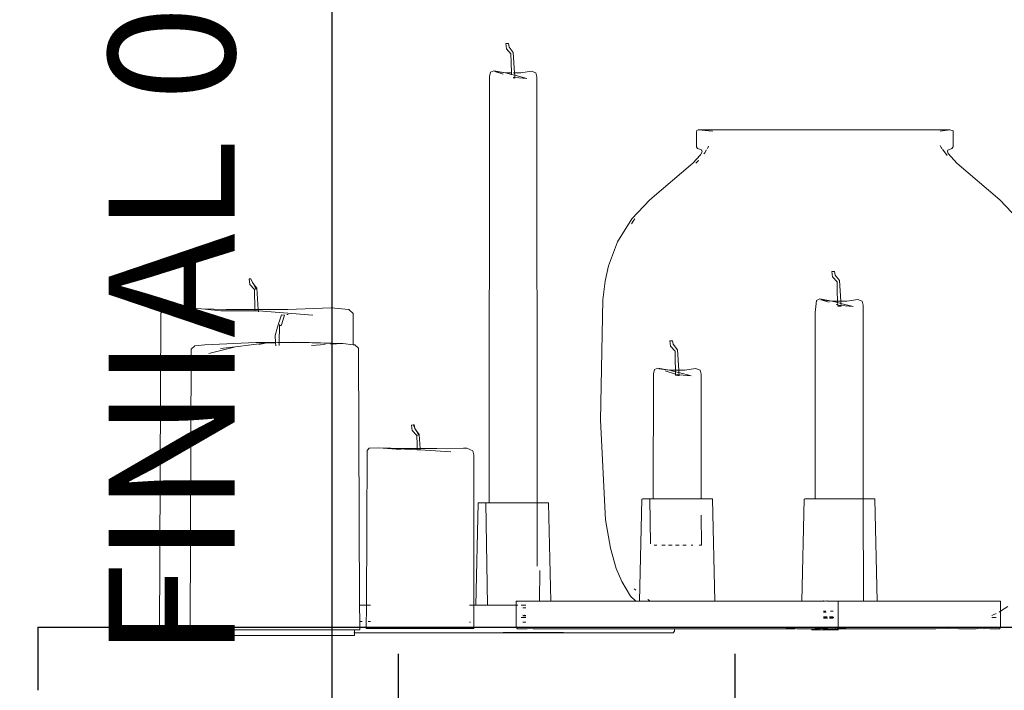
# Model space of a CAD drawing. Units: millimetres. Extents: x 7894 to 8038, y 6851 to 6951.
# Tile 45 of 49: x 7942.814 to 7950.619, y 6936.88 to 6942.195. Entities that reach past the tile are written whole.
import ezdxf

# ---------------------------------------------------------------- set-up
doc = ezdxf.new("R2010")
doc.units = ezdxf.units.MM
for name, color, linetype, lineweight in [('A-ANNO-DIMS', 2, 'Continuous', 18), ('A-FURN-ACCS', 8, 'Continuous', 13), ('A-FURN-SHLF', 7, 'Continuous', 30)]:
    doc.layers.add(name, color=color, linetype=linetype, lineweight=lineweight)
doc.styles.get("Standard").update_dxf_attribs({"font": 'arial.ttf'})
doc.dimstyles.new('ISO-25', dxfattribs={"dimtxt": 1, "dimasz": 1, "dimexe": 1.25, "dimexo": 0.625, "dimtad": 1, "dimdec": 0, "dimlunit": 4, "dimtxsty": 'Standard', "dimcen": 2.5, "dimclrt": 1, "dimadec": 0, "dimazin": 0, "dimtfac": 1, "dimtdec": 0, "dimtmove": 0, "dimatfit": 3, "dimfxl": 1, "dimarcsym": 0})

# ---------------------------------------------------------------- blocks, each defined once
blk = doc.blocks.new('FLOATING-SHELF-ELEV')
for q in [(17.3035, 0.5), (0, 0)]:
    blk.add_line((0, 0.5), q)
blk = doc.blocks.new('*D17')
at = {"layer": 'A-ANNO-DIMS', "color": 0, "lineweight": -2, "transparency": 16777216}
for p, q in [((7945.2906, 6935.3937), (7945.2906, 6950.7481)), ((7945.1919, 6935.3937), (7944.0406, 6935.3937)), ((7945.2906, 6932.8853), (7945.2906, 6934.3937)), ((7945.1919, 6931.8853), (7944.0406, 6931.8853))]:
    blk.add_line(p, q, dxfattribs=at)
at = {"layer": 'A-ANNO-DIMS', "color": 0, "transparency": 16777216}
for points in [[(7945.124, 6934.3937), (7945.4573, 6934.3937), (7945.2906, 6935.3937)], [(7945.124, 6932.8853), (7945.4573, 6932.8853), (7945.2906, 6931.8853)]]:
    blk.add_solid(points, dxfattribs=at)
at = {"layer": 'Defpoints', "color": 0, "transparency": 16777216}
for p in [(7945.2906, 6935.3937), (7945.8169, 6935.3937), (7945.8169, 6931.8853)]:
    blk.add_point(p, dxfattribs=at)
at = {"layer": 'A-ANNO-DIMS', "color": 1, "transparency": 16777216, "insert": (7944.1482, 6943.5709), "char_height": 1, "attachment_point": 5, "rotation": 90}
blk.add_mtext('FINIAL 0\'-3 1/2" TYP.', dxfattribs=at)
blk = doc.blocks.new('*D18')
at = {"layer": 'A-ANNO-DIMS', "color": 0, "lineweight": -2, "transparency": 16777216}
for p, q in [((7945.8169, 6936.0187), (7945.8169, 6937.17)), ((7948.487, 6936.0187), (7948.487, 6937.17)), ((7944.8169, 6935.92), (7943.8169, 6935.92)), ((7945.8169, 6935.92), (7948.487, 6935.92)), ((7949.487, 6935.92), (7960.1626, 6935.92))]:
    blk.add_line(p, q, dxfattribs=at)
at = {"layer": 'A-ANNO-DIMS', "color": 0, "transparency": 16777216}
for points in [[(7944.8169, 6936.0867), (7944.8169, 6935.7534), (7945.8169, 6935.92)], [(7949.487, 6936.0867), (7949.487, 6935.7534), (7948.487, 6935.92)]]:
    blk.add_solid(points, dxfattribs=at)
at = {"layer": 'Defpoints', "color": 0, "transparency": 16777216}
for p in [(7948.487, 6935.92), (7945.8169, 6935.3937), (7948.487, 6935.3937)]:
    blk.add_point(p, dxfattribs=at)
at = {"layer": 'A-ANNO-DIMS', "color": 1, "transparency": 16777216, "insert": (7955.3248, 6937.0621), "char_height": 1, "attachment_point": 5}
blk.add_mtext('0\'-2 1/2" TYP.', dxfattribs=at)
blk = doc.blocks.new('*D23')
at = {"layer": 'A-ANNO-DIMS', "color": 0, "lineweight": -2, "transparency": 16777216}
for p, q in [((7940.0888, 6907.098), (7940.0888, 6947.7928)), ((7971.9356, 6928.989), (7971.9356, 6947.7928)), ((7941.0888, 6946.5428), (7970.9356, 6946.5428))]:
    blk.add_line(p, q, dxfattribs=at)
at = {"layer": 'A-ANNO-DIMS', "color": 0, "transparency": 16777216}
for points in [[(7941.0888, 6946.7095), (7941.0888, 6946.3762), (7940.0888, 6946.5428)], [(7970.9356, 6946.7095), (7970.9356, 6946.3762), (7971.9356, 6946.5428)]]:
    blk.add_solid(points, dxfattribs=at)
at = {"layer": 'Defpoints', "color": 0, "transparency": 16777216}
for p in [(7971.9356, 6946.5428), (7971.9356, 6928.364), (7940.0888, 6906.473)]:
    blk.add_point(p, dxfattribs=at)
at = {"layer": 'A-ANNO-DIMS', "color": 1, "transparency": 16777216, "insert": (7956.0122, 6947.6784), "char_height": 1, "attachment_point": 5}
blk.add_mtext('2\'-8"', dxfattribs=at)
blk = doc.blocks.new('*D24')
at = {"layer": 'A-ANNO-DIMS', "color": 0, "lineweight": -2, "transparency": 16777216}
for p, q in [((7953.3408, 6944.6059), (7936.9023, 6944.6059)), ((7938.1523, 6907.473), (7938.1523, 6943.6059)), ((7939.4638, 6906.473), (7936.9023, 6906.473))]:
    blk.add_line(p, q, dxfattribs=at)
at = {"layer": 'A-ANNO-DIMS', "color": 0, "transparency": 16777216}
for points in [[(7937.9856, 6943.6059), (7938.319, 6943.6059), (7938.1523, 6944.6059)], [(7937.9856, 6907.473), (7938.319, 6907.473), (7938.1523, 6906.473)]]:
    blk.add_solid(points, dxfattribs=at)
at = {"layer": 'Defpoints', "color": 0, "transparency": 16777216}
for p in [(7938.1523, 6944.6059), (7953.9658, 6944.6059), (7940.0888, 6906.473)]:
    blk.add_point(p, dxfattribs=at)
at = {"layer": 'A-ANNO-DIMS', "color": 1, "transparency": 16777216, "insert": (7937.0164, 6925.5395), "char_height": 1, "attachment_point": 5, "rotation": 90}
blk.add_mtext('3\'-2"', dxfattribs=at)

msp = doc.modelspace()

# ---------------------------------------------------------------- linework, layer by layer
at = {"layer": 'A-FURN-ACCS'}
for p, q in [((7946.6885, 6942.0066), (7946.6676, 6942.0055)), ((7946.6728, 6941.9643), (7946.6676, 6942.0055)), ((7946.708, 6941.9254), (7946.6728, 6941.9643)), ((7946.6933, 6941.9783), (7946.6885, 6942.0066)), ((7946.7263, 6941.9342), (7946.6933, 6941.9783)), ((7946.7263, 6941.9342), (7946.737, 6941.7738)), ((7946.7095, 6941.8548), (7946.708, 6941.9254)), ((7946.7117, 6941.7739), (7946.7095, 6941.8548)), ((7946.5382, 6941.7452), (7946.5461, 6941.7792)), ((7946.5719, 6941.7913), (7946.5461, 6941.7792)), ((7946.6654, 6941.7739), (7946.5719, 6941.7913)), ((7946.6468, 6941.764), (7946.5806, 6941.7848)), ((7946.5806, 6941.7848), (7946.6654, 6941.7739)), ((7946.7855, 6941.7738), (7946.8704, 6941.7866)), ((7946.8704, 6941.7866), (7946.9048, 6941.7734)), ((7946.536, 6938.3656), (7946.5382, 6941.7452)), ((7946.6654, 6941.7739), (7946.7117, 6941.7739)), ((7946.712, 6941.7619), (7946.6654, 6941.7739)), ((7946.712, 6941.7619), (7946.7117, 6941.7739)), ((7946.7383, 6941.7551), (7946.712, 6941.7619)), ((7946.7121, 6941.7574), (7946.712, 6941.7619)), ((7946.7294, 6941.7334), (7946.7255, 6941.7336)), ((7946.7282, 6941.7738), (7946.7356, 6941.7738)), ((7946.7293, 6941.7391), (7946.7394, 6941.7382)), ((7946.7294, 6941.7334), (7946.7398, 6941.7331)), ((7946.737, 6941.7738), (7946.7855, 6941.7738)), ((7946.737, 6941.7738), (7946.7383, 6941.7551)), ((7946.834, 6941.7303), (7946.7383, 6941.7551)), ((7946.7383, 6941.7551), (7946.7391, 6941.7429)), ((7946.7394, 6941.7382), (7946.7398, 6941.7331)), ((7946.7394, 6941.7382), (7946.834, 6941.7303)), ((7946.9048, 6941.7734), (7946.9128, 6941.7428)), ((7946.9151, 6938.3656), (7946.9128, 6941.7428)), ((7948.1826, 6941.3166), (7948.1783, 6941.3073)), ((7948.1932, 6941.3214), (7948.1826, 6941.3166)), ((7948.2264, 6941.3214), (7948.1932, 6941.3214)), ((7948.1932, 6941.3214), (7948.2768, 6941.3155)), ((7948.2335, 6941.322), (7948.2264, 6941.3214)), ((7948.2335, 6941.322), (7948.3411, 6941.322)), ((7948.2768, 6941.3155), (7948.2776, 6941.315)), ((7948.2776, 6941.315), (7948.282, 6941.3123)), ((7948.2776, 6941.315), (7948.3047, 6941.3129)), ((7948.3047, 6941.3129), (7948.3061, 6941.3129)), ((7948.4842, 6941.3214), (7948.3411, 6941.322)), ((7948.4842, 6941.3214), (7948.6983, 6941.3214)), ((7948.6983, 6941.3214), (7948.9364, 6941.322)), ((7948.9364, 6941.322), (7948.9403, 6941.322)), ((7948.9403, 6941.322), (7948.9441, 6941.322)), ((7948.9441, 6941.322), (7949.1925, 6941.3214)), ((7949.46, 6941.3214), (7949.1925, 6941.3214)), ((7949.688, 6941.322), (7949.46, 6941.3214)), ((7949.6989, 6941.322), (7949.688, 6941.322)), ((7949.6989, 6941.322), (7949.8994, 6941.322)), ((7950.0634, 6941.3214), (7949.8994, 6941.322)), ((7950.0634, 6941.3214), (7950.1666, 6941.3214)), ((7950.1103, 6941.3124), (7950.1865, 6941.322)), ((7950.1666, 6941.3214), (7950.1865, 6941.322)), ((7950.1865, 6941.322), (7950.2129, 6941.3132)), ((7950.2129, 6941.3132), (7950.2128, 6941.1884)), ((7948.1802, 6941.1884), (7948.1783, 6941.3073)), ((7948.1802, 6941.1884), (7948.1875, 6941.1754)), ((7948.1875, 6941.1754), (7948.2202, 6941.1628)), ((7948.2202, 6941.1628), (7948.2242, 6941.1488)), ((7948.2454, 6941.1398), (7948.2596, 6941.1648)), ((7948.2658, 6941.1757), (7948.2755, 6941.1928)), ((7950.1181, 6941.1829), (7950.1105, 6941.1991)), ((7950.1245, 6941.1748), (7950.1181, 6941.1829)), ((7950.1678, 6941.1195), (7950.1291, 6941.1689)), ((7950.1713, 6941.1615), (7950.1683, 6941.1541)), ((7950.1683, 6941.1541), (7950.175, 6941.1344)), ((7950.204, 6941.1742), (7950.1713, 6941.1615)), ((7950.2128, 6941.1884), (7950.204, 6941.1742)), ((7948.2118, 6941.1249), (7948.151, 6941.0589)), ((7948.1731, 6941.0589), (7948.1914, 6941.0764)), ((7948.196, 6941.0819), (7948.1914, 6941.0764)), ((7948.2242, 6941.1488), (7948.2118, 6941.1249)), ((7948.2454, 6941.1398), (7948.238, 6941.131)), ((7950.175, 6941.1344), (7950.242, 6941.0589)), ((7948.151, 6941.0589), (7947.8087, 6940.7689)), ((7950.242, 6941.0589), (7950.5843, 6940.7689)), ((7947.8087, 6940.7689), (7947.6662, 6940.6157)), ((7950.5843, 6940.7689), (7950.7268, 6940.6157)), ((7947.6662, 6940.6157), (7947.5524, 6940.4339)), ((7947.6819, 6940.6052), (7947.6907, 6940.6157)), ((7947.6632, 6940.5777), (7947.6819, 6940.6052)), ((7947.5524, 6940.4339), (7947.4814, 6940.2451)), ((7947.4814, 6940.2451), (7947.4545, 6940.1238)), ((7944.6329, 6940.1404), (7944.6464, 6940.1411)), ((7944.6329, 6940.1404), (7944.6384, 6940.0978)), ((7944.6598, 6940.1124), (7944.6464, 6940.1411)), ((7949.2744, 6940.2), (7949.2533, 6940.1989)), ((7949.2585, 6940.1573), (7949.2533, 6940.1989)), ((7949.2941, 6940.1181), (7949.2585, 6940.1573)), ((7949.2792, 6940.1714), (7949.2744, 6940.2)), ((7949.3124, 6940.127), (7949.2792, 6940.1714)), ((7944.6384, 6940.0978), (7944.6751, 6940.0572)), ((7944.6647, 6940.1057), (7944.6598, 6940.1124)), ((7944.6941, 6940.0665), (7944.6647, 6940.1057)), ((7944.687, 6940.0629), (7944.6647, 6940.1057)), ((7944.6751, 6940.0572), (7944.687, 6940.0629)), ((7944.687, 6940.0629), (7944.6941, 6940.0665)), ((7944.7053, 6939.8994), (7944.6941, 6940.0665)), ((7947.4545, 6940.1238), (7947.4357, 6939.9752)), ((7949.2956, 6940.0469), (7949.2941, 6940.1181)), ((7949.3124, 6940.127), (7949.3233, 6939.9651)), ((7944.6751, 6940.0572), (7944.679, 6939.8994)), ((7949.1568, 6939.9828), (7949.1308, 6939.9707)), ((7949.1568, 6939.9828), (7949.2511, 6939.9649)), ((7949.2977, 6939.965), (7949.2956, 6940.0469)), ((7943.934, 6939.8696), (7943.9664, 6939.905)), ((7943.9664, 6939.905), (7944.0713, 6939.9175)), ((7944.0713, 6939.9175), (7944.2541, 6939.9024)), ((7945.2843, 6939.9127), (7944.9393, 6939.8993)), ((7945.2843, 6939.9127), (7945.4243, 6939.8989)), ((7947.4357, 6939.9752), (7947.4184, 6939.0212)), ((7949.1201, 6939.8758), (7949.1308, 6939.9707)), ((7949.1656, 6939.9763), (7949.2511, 6939.9649)), ((7949.2323, 6939.9554), (7949.1656, 6939.9763)), ((7949.2977, 6939.965), (7949.2511, 6939.9649)), ((7949.2981, 6939.9529), (7949.2511, 6939.9649)), ((7949.2985, 6939.9346), (7949.2855, 6939.9387)), ((7949.3233, 6939.9651), (7949.2977, 6939.965)), ((7949.2981, 6939.9529), (7949.2977, 6939.965)), ((7949.2982, 6939.9487), (7949.2981, 6939.9529)), ((7949.3246, 6939.9461), (7949.2981, 6939.9529)), ((7949.2985, 6939.9346), (7949.2983, 6939.9429)), ((7949.3117, 6939.9305), (7949.2985, 6939.9346)), ((7949.2988, 6939.9254), (7949.2985, 6939.9346)), ((7949.3157, 6939.9245), (7949.2988, 6939.9254)), ((7949.3257, 6939.9293), (7949.3117, 6939.9305)), ((7949.3157, 6939.9245), (7949.3261, 6939.9242)), ((7949.3722, 6939.9652), (7949.3233, 6939.9651)), ((7949.3233, 6939.9651), (7949.3246, 6939.9461)), ((7949.3246, 6939.9461), (7949.3254, 6939.9342)), ((7949.4211, 6939.9213), (7949.3246, 6939.9461)), ((7949.3257, 6939.9293), (7949.3261, 6939.9242)), ((7949.4211, 6939.9213), (7949.3257, 6939.9293)), ((7949.4578, 6939.9781), (7949.3722, 6939.9652)), ((7949.4925, 6939.9648), (7949.4578, 6939.9781)), ((7949.5005, 6939.934), (7949.4925, 6939.9648)), ((7949.5017, 6938.3978), (7949.5005, 6939.934)), ((7943.9233, 6937.3141), (7943.934, 6939.8696)), ((7944.2541, 6939.9024), (7944.4514, 6939.8995)), ((7944.2541, 6939.9024), (7944.4087, 6939.8888)), ((7944.4087, 6939.8888), (7944.4173, 6939.8887)), ((7944.4173, 6939.8887), (7944.6793, 6939.8885)), ((7944.4514, 6939.8995), (7944.679, 6939.8994)), ((7944.679, 6939.8994), (7944.6793, 6939.8885)), ((7944.6793, 6939.8885), (7944.6954, 6939.8885)), ((7944.6846, 6939.8994), (7944.7053, 6939.8994)), ((7944.6954, 6939.8885), (7944.7061, 6939.8876)), ((7944.7053, 6939.8994), (7944.9393, 6939.8993)), ((7944.7061, 6939.8876), (7944.7053, 6939.8994)), ((7944.7061, 6939.8876), (7945.1366, 6939.854)), ((7944.7067, 6939.8797), (7944.7061, 6939.8876)), ((7944.8619, 6939.7764), (7944.8901, 6939.8551)), ((7944.8889, 6939.7764), (7944.9126, 6939.8547)), ((7944.8901, 6939.8551), (7944.9126, 6939.8547)), ((7944.9315, 6939.8584), (7944.9431, 6939.8582)), ((7945.4567, 6939.8671), (7945.4243, 6939.8989)), ((7945.4577, 6939.619), (7945.4567, 6939.8671)), ((7949.1201, 6938.3978), (7949.1201, 6939.8758)), ((7944.8398, 6939.6934), (7944.8619, 6939.7764)), ((7944.8736, 6939.7707), (7944.8705, 6939.6381)), ((7944.8746, 6939.78), (7944.8736, 6939.7707)), ((7944.8736, 6939.7707), (7944.8855, 6939.7707)), ((7944.8855, 6939.7707), (7944.8889, 6939.7764)), ((7944.843, 6939.6381), (7944.8398, 6939.6934)), ((7944.2022, 6939.6117), (7944.174, 6939.583)), ((7944.2812, 6939.6187), (7944.2022, 6939.6117)), ((7944.6857, 6939.638), (7944.2812, 6939.6187)), ((7944.3123, 6939.5507), (7944.5251, 6939.6017)), ((7944.4069, 6939.5882), (7944.5251, 6939.6017)), ((7944.7722, 6939.6332), (7944.5251, 6939.6017)), ((7944.6857, 6939.638), (7944.843, 6939.6381)), ((7944.7097, 6939.622), (7944.7722, 6939.6332)), ((7944.7722, 6939.6332), (7944.8431, 6939.6353)), ((7944.843, 6939.6381), (7944.8455, 6939.6381)), ((7944.8431, 6939.6353), (7944.843, 6939.6381)), ((7944.8431, 6939.6353), (7944.8704, 6939.6361)), ((7944.8446, 6939.6105), (7944.8431, 6939.6353)), ((7944.8597, 6939.6381), (7944.8705, 6939.6381)), ((7944.8704, 6939.6361), (7944.8698, 6939.6137)), ((7944.8704, 6939.6361), (7944.9366, 6939.6381)), ((7944.8705, 6939.6381), (7944.8704, 6939.6361)), ((7944.8705, 6939.6381), (7944.9366, 6939.6381)), ((7944.9366, 6939.6381), (7944.9883, 6939.6397)), ((7944.9366, 6939.6381), (7945.0318, 6939.6382)), ((7944.9883, 6939.6397), (7945.0318, 6939.6382)), ((7945.0318, 6939.6382), (7945.3246, 6939.628)), ((7945.0318, 6939.6382), (7945.1106, 6939.6382)), ((7945.1106, 6939.6382), (7945.3753, 6939.6281)), ((7945.1265, 6939.6135), (7945.2348, 6939.6199)), ((7945.2788, 6939.6225), (7945.3753, 6939.6281)), ((7945.3753, 6939.6281), (7945.3246, 6939.628)), ((7945.3753, 6939.6281), (7945.4577, 6939.619)), ((7945.4577, 6939.619), (7945.4719, 6939.6191)), ((7945.4719, 6939.6191), (7945.5, 6939.5908)), ((7945.5, 6939.5908), (7945.5086, 6937.5546)), ((7947.9897, 6939.6512), (7947.9686, 6939.65)), ((7947.9739, 6939.6086), (7947.9686, 6939.65)), ((7948.0093, 6939.5694), (7947.9739, 6939.6086)), ((7947.9945, 6939.6227), (7947.9897, 6939.6512)), ((7948.0277, 6939.5784), (7947.9945, 6939.6227)), ((7944.1646, 6937.3606), (7944.174, 6939.583)), ((7948.0108, 6939.4984), (7948.0093, 6939.5694)), ((7948.0277, 6939.5784), (7948.0385, 6939.4169)), ((7948.013, 6939.417), (7948.0108, 6939.4984)), ((7947.8365, 6938.3978), (7947.8384, 6939.3882)), ((7947.8384, 6939.3882), (7947.8464, 6939.4223)), ((7947.8464, 6939.4223), (7947.8724, 6939.4345)), ((7947.8724, 6939.4345), (7947.9665, 6939.417)), ((7947.8811, 6939.428), (7947.9665, 6939.417)), ((7947.9301, 6939.4126), (7948.0138, 6939.3864)), ((7947.9665, 6939.417), (7948.013, 6939.417)), ((7947.9665, 6939.417), (7948.0133, 6939.4049)), ((7948.013, 6939.417), (7948.0385, 6939.4169)), ((7948.0133, 6939.4049), (7948.013, 6939.417)), ((7948.0133, 6939.4049), (7948.0398, 6939.3981)), ((7948.0138, 6939.3864), (7948.0133, 6939.4049)), ((7948.0138, 6939.3864), (7948.0269, 6939.3823)), ((7948.014, 6939.3771), (7948.0138, 6939.3864)), ((7948.0309, 6939.3762), (7948.014, 6939.3771)), ((7948.0409, 6939.3811), (7948.0269, 6939.3823)), ((7948.0309, 6939.3762), (7948.0413, 6939.376)), ((7948.0385, 6939.4169), (7948.0873, 6939.4169)), ((7948.0385, 6939.4169), (7948.0398, 6939.3981)), ((7948.0398, 6939.3981), (7948.1361, 6939.3731)), ((7948.0398, 6939.3981), (7948.0409, 6939.3811)), ((7948.1361, 6939.3731), (7948.0409, 6939.3811)), ((7948.0409, 6939.3811), (7948.0413, 6939.376)), ((7948.0873, 6939.4169), (7948.1727, 6939.4298)), ((7948.2074, 6939.4165), (7948.1727, 6939.4298)), ((7948.2154, 6939.3857), (7948.2074, 6939.4165)), ((7948.2154, 6939.3857), (7948.2173, 6938.3978)), ((7945.9339, 6938.9834), (7945.9202, 6938.9823)), ((7945.9257, 6938.9396), (7945.9202, 6938.9823)), ((7945.9339, 6938.9834), (7945.9421, 6938.9837)), ((7945.9463, 6938.9592), (7945.9339, 6938.9834)), ((7945.9463, 6938.9592), (7945.9421, 6938.9837)), ((7947.4184, 6939.0212), (7947.4584, 6938.2318)), ((7945.9257, 6938.9396), (7945.9625, 6938.8991)), ((7945.9471, 6938.9542), (7945.9463, 6938.9592)), ((7945.9527, 6938.9468), (7945.9463, 6938.9592)), ((7945.9527, 6938.9468), (7945.9471, 6938.9542)), ((7945.9743, 6938.9047), (7945.9527, 6938.9468)), ((7945.9815, 6938.9083), (7945.9527, 6938.9468)), ((7945.9743, 6938.9047), (7945.9625, 6938.8991)), ((7945.9642, 6938.8272), (7945.9625, 6938.8991)), ((7945.9815, 6938.9083), (7945.9743, 6938.9047)), ((7945.989, 6938.7964), (7945.9815, 6938.9083)), ((7945.964, 6938.8255), (7945.9642, 6938.8272)), ((7945.964, 6938.8255), (7945.9648, 6938.7964)), ((7945.5621, 6937.5546), (7945.5673, 6938.78)), ((7945.5673, 6938.78), (7945.5851, 6938.7995)), ((7945.6624, 6938.8027), (7945.5851, 6938.7995)), ((7945.8333, 6938.789), (7945.6624, 6938.8027)), ((7945.8527, 6938.7965), (7945.6624, 6938.8027)), ((7945.6624, 6938.8027), (7945.9651, 6938.7868)), ((7945.9648, 6938.7964), (7945.8527, 6938.7965)), ((7945.9648, 6938.7964), (7945.9651, 6938.7868)), ((7945.989, 6938.7964), (7945.9648, 6938.7964)), ((7945.9651, 6938.7868), (7945.9873, 6938.7862)), ((7945.9897, 6938.7859), (7945.9873, 6938.7862)), ((7945.9897, 6938.7859), (7945.989, 6938.7964)), ((7946.1219, 6938.7964), (7945.989, 6938.7964)), ((7946.2307, 6938.7714), (7945.9897, 6938.7859)), ((7945.991, 6938.7671), (7945.9909, 6938.7682)), ((7946.3315, 6938.7997), (7946.1219, 6938.7964)), ((7946.3577, 6938.7984), (7946.3315, 6938.7997)), ((7946.4073, 6938.7786), (7946.3577, 6938.7984)), ((7946.4132, 6938.7456), (7946.4073, 6938.7786)), ((7946.4132, 6938.7456), (7946.4132, 6937.5546)), ((7946.4299, 6937.5546), (7946.4485, 6938.3628)), ((7946.4485, 6938.3628), (7946.4517, 6938.3656)), ((7946.4681, 6938.3656), (7946.4517, 6938.3656)), ((7946.473, 6938.3656), (7946.4681, 6938.3656)), ((7946.4773, 6938.3656), (7946.473, 6938.3656)), ((7946.4786, 6938.3656), (7946.4773, 6938.3656)), ((7946.4802, 6938.3656), (7946.4786, 6938.3656)), ((7946.4899, 6938.3656), (7946.4802, 6938.3656)), ((7946.4899, 6938.3656), (7946.4994, 6938.3656)), ((7946.4994, 6938.3656), (7946.5044, 6938.3656)), ((7946.5044, 6938.3656), (7946.5068, 6938.3656)), ((7946.5068, 6938.3656), (7946.5105, 6938.3656)), ((7946.5105, 6938.3656), (7946.5224, 6937.5546)), ((7946.5105, 6938.3656), (7946.5165, 6938.3656)), ((7946.522, 6938.3656), (7946.5165, 6938.3656)), ((7946.5233, 6938.3656), (7946.522, 6938.3656)), ((7946.536, 6938.3656), (7946.5233, 6938.3656)), ((7946.536, 6938.3656), (7946.5418, 6938.3656)), ((7946.536, 6938.3628), (7946.536, 6938.3656)), ((7946.5418, 6938.3656), (7946.5434, 6938.3656)), ((7946.5434, 6938.3656), (7946.551, 6938.3656)), ((7946.551, 6938.3656), (7946.5537, 6938.3656)), ((7946.5537, 6938.3656), (7946.5557, 6938.3656)), ((7946.5557, 6938.3656), (7946.566, 6938.3656)), ((7946.5725, 6938.3656), (7946.566, 6938.3656)), ((7946.5725, 6938.3656), (7946.5825, 6938.3656)), ((7946.5844, 6938.3656), (7946.5825, 6938.3656)), ((7946.5862, 6938.3656), (7946.5844, 6938.3656)), ((7946.5871, 6938.3656), (7946.5862, 6938.3656)), ((7946.5885, 6938.3656), (7946.5871, 6938.3656)), ((7946.5915, 6938.3656), (7946.5885, 6938.3656)), ((7946.5915, 6938.3656), (7946.5991, 6938.3656)), ((7946.6111, 6938.3656), (7946.5991, 6938.3656)), ((7946.6111, 6938.3656), (7946.6358, 6938.3656)), ((7946.6623, 6938.3656), (7946.6358, 6938.3656)), ((7946.6623, 6938.3656), (7946.676, 6938.3656)), ((7946.676, 6938.3656), (7946.7159, 6938.3656)), ((7946.7159, 6938.3656), (7946.7182, 6938.3656)), ((7946.7182, 6938.3656), (7946.7396, 6938.3656)), ((7946.7431, 6938.3656), (7946.7396, 6938.3656)), ((7946.7431, 6938.3656), (7946.7818, 6938.3656)), ((7946.7966, 6938.3656), (7946.7818, 6938.3656)), ((7946.7966, 6938.3656), (7946.8219, 6938.3656)), ((7946.8475, 6938.3656), (7946.8219, 6938.3656)), ((7946.8475, 6938.3656), (7946.8584, 6938.3656)), ((7946.8584, 6938.3656), (7946.8714, 6938.3656)), ((7946.8714, 6938.3656), (7946.8898, 6938.3656)), ((7946.8898, 6938.3656), (7946.8943, 6938.3656)), ((7946.9059, 6938.3656), (7946.8943, 6938.3656)), ((7946.9059, 6938.3656), (7946.912, 6938.3656)), ((7946.912, 6938.3656), (7946.9151, 6938.3656)), ((7946.9152, 6937.8652), (7946.9151, 6938.3656)), ((7946.9167, 6938.3656), (7946.9151, 6938.3656)), ((7946.9224, 6938.3656), (7946.9167, 6938.3656)), ((7946.9233, 6938.3656), (7946.9224, 6938.3656)), ((7946.9242, 6938.3656), (7946.9233, 6938.3656)), ((7946.9242, 6938.3656), (7946.9251, 6938.3656)), ((7946.9279, 6938.3656), (7946.9251, 6938.3656)), ((7946.9288, 6938.3656), (7946.9279, 6938.3656)), ((7946.9303, 6938.3656), (7946.9288, 6938.3656)), ((7946.9317, 6938.3656), (7946.9303, 6938.3656)), ((7946.9338, 6938.3656), (7946.9317, 6938.3656)), ((7946.9361, 6938.3656), (7946.9338, 6938.3656)), ((7946.9371, 6938.3656), (7946.9361, 6938.3656)), ((7946.9371, 6938.3656), (7946.9392, 6938.3656)), ((7946.9379, 6938.3656), (7946.9371, 6938.3656)), ((7946.9392, 6938.3656), (7946.9379, 6938.3656)), ((7946.9392, 6938.3656), (7946.9408, 6938.3656)), ((7946.943, 6938.3656), (7946.9408, 6938.3656)), ((7946.9453, 6938.3656), (7946.943, 6938.3656)), ((7946.9453, 6938.3656), (7946.9453, 6938.3628)), ((7946.9474, 6938.3656), (7946.9453, 6938.3656)), ((7946.949, 6938.3656), (7946.9474, 6938.3656)), ((7946.9598, 6938.3656), (7946.949, 6938.3656)), ((7946.9637, 6938.3656), (7946.9598, 6938.3656)), ((7946.9659, 6938.3656), (7946.9637, 6938.3656)), ((7946.9671, 6938.3656), (7946.9659, 6938.3656)), ((7946.9671, 6938.3656), (7947.004, 6938.3656)), ((7947.0073, 6938.3628), (7947.004, 6938.3656)), ((7947.0252, 6937.5869), (7947.0073, 6938.3628)), ((7947.7285, 6937.5869), (7947.7471, 6938.3951)), ((7947.7471, 6938.3951), (7947.7505, 6938.3978)), ((7947.7505, 6938.3978), (7947.7838, 6938.3979)), ((7947.7838, 6938.3979), (7947.7867, 6938.3979)), ((7947.7867, 6938.3979), (7947.7886, 6938.3978)), ((7947.7886, 6938.3978), (7947.7902, 6938.3978)), ((7947.7902, 6938.3978), (7947.791, 6938.3979)), ((7947.791, 6938.3979), (7947.7955, 6938.3979)), ((7947.7955, 6938.3979), (7947.8035, 6938.3978)), ((7947.8035, 6938.3978), (7947.8048, 6938.3979)), ((7947.8048, 6938.3979), (7947.8066, 6938.3979)), ((7947.8066, 6938.3979), (7947.8092, 6938.3979)), ((7947.8092, 6938.3979), (7947.8144, 6938.0417)), ((7947.8092, 6938.3979), (7947.8157, 6938.3979)), ((7947.8157, 6938.3979), (7947.8228, 6938.3978)), ((7947.8228, 6938.3978), (7947.8294, 6938.3979)), ((7947.8294, 6938.3979), (7947.8303, 6938.3979)), ((7947.8353, 6938.3979), (7947.8303, 6938.3979)), ((7947.8365, 6938.3978), (7947.8353, 6938.3979)), ((7947.8365, 6938.3951), (7947.8365, 6938.3978)), ((7947.8365, 6938.3978), (7947.8515, 6938.3978)), ((7947.8515, 6938.3978), (7947.8524, 6938.3979)), ((7947.8524, 6938.3979), (7947.8812, 6938.3979)), ((7947.8858, 6938.3978), (7947.8812, 6938.3979)), ((7947.8858, 6938.3978), (7947.8977, 6938.3979)), ((7947.9609, 6938.3978), (7947.8977, 6938.3979)), ((7947.9609, 6938.3978), (7947.9747, 6938.3979)), ((7948.0146, 6938.3978), (7947.9747, 6938.3979)), ((7948.0146, 6938.3978), (7948.0169, 6938.3979)), ((7948.0169, 6938.3979), (7948.0383, 6938.3979)), ((7948.0417, 6938.3978), (7948.0383, 6938.3979)), ((7948.0417, 6938.3978), (7948.0804, 6938.3979)), ((7948.0953, 6938.3978), (7948.0804, 6938.3979)), ((7948.157, 6938.3979), (7948.0953, 6938.3978)), ((7948.157, 6938.3979), (7948.1701, 6938.3978)), ((7948.1701, 6938.3978), (7948.1735, 6938.3979)), ((7948.1735, 6938.3979), (7948.2022, 6938.3978)), ((7948.2022, 6938.3978), (7948.2173, 6938.3978)), ((7948.2173, 6938.3978), (7948.2173, 6938.3951)), ((7948.2325, 6938.3978), (7948.2173, 6938.3978)), ((7948.2325, 6938.3978), (7948.2341, 6938.3979)), ((7948.2341, 6938.3979), (7948.2354, 6938.3979)), ((7948.2354, 6938.3979), (7948.2417, 6938.3979)), ((7948.244, 6938.3979), (7948.2417, 6938.3979)), ((7948.244, 6938.3979), (7948.2439, 6938.3951)), ((7948.2629, 6938.3978), (7948.244, 6938.3979)), ((7948.2629, 6938.3978), (7948.2645, 6938.3978)), ((7948.2683, 6938.3979), (7948.2645, 6938.3978)), ((7948.2758, 6938.3978), (7948.2683, 6938.3979)), ((7948.2758, 6938.3978), (7948.3028, 6938.3978)), ((7948.306, 6938.3951), (7948.3028, 6938.3978)), ((7948.3246, 6937.5869), (7948.306, 6938.3951)), ((7949.0151, 6937.5869), (7949.0337, 6938.3951)), ((7949.0337, 6938.3951), (7949.0371, 6938.3978)), ((7949.0371, 6938.3978), (7949.0707, 6938.3978)), ((7949.0737, 6938.3979), (7949.0707, 6938.3978)), ((7949.086, 6938.3979), (7949.0737, 6938.3979)), ((7949.0901, 6938.3978), (7949.086, 6938.3979)), ((7949.092, 6938.3978), (7949.0901, 6938.3978)), ((7949.0958, 6938.3979), (7949.092, 6938.3978)), ((7949.0958, 6938.3979), (7949.1023, 6938.3979)), ((7949.0958, 6938.3979), (7949.0958, 6938.3951)), ((7949.1072, 6938.3978), (7949.1023, 6938.3979)), ((7949.111, 6938.3979), (7949.1072, 6938.3978)), ((7949.116, 6938.3979), (7949.111, 6938.3979)), ((7949.1169, 6938.3979), (7949.116, 6938.3979)), ((7949.1201, 6938.3978), (7949.1169, 6938.3979)), ((7949.126, 6938.3979), (7949.1201, 6938.3978)), ((7949.1201, 6938.3951), (7949.1201, 6938.3978)), ((7949.1287, 6938.3978), (7949.126, 6938.3979)), ((7949.1287, 6938.3978), (7949.1324, 6938.3979)), ((7949.1324, 6938.3979), (7949.1362, 6938.3978)), ((7949.1362, 6938.3978), (7949.139, 6938.3979)), ((7949.139, 6938.3979), (7949.1497, 6938.3978)), ((7949.1497, 6938.3978), (7949.1526, 6938.3979)), ((7949.1526, 6938.3979), (7949.1762, 6938.3978)), ((7949.1762, 6938.3978), (7949.1827, 6938.3979)), ((7949.1827, 6938.3979), (7949.1843, 6938.3979)), ((7949.1964, 6938.3978), (7949.1843, 6938.3979)), ((7949.1964, 6938.3978), (7949.2021, 6938.3979)), ((7949.2144, 6938.3978), (7949.2021, 6938.3979)), ((7949.2144, 6938.3978), (7949.2408, 6938.3979)), ((7949.2475, 6938.3978), (7949.2408, 6938.3979)), ((7949.2475, 6938.3978), (7949.2822, 6938.3979)), ((7949.3012, 6938.3978), (7949.2822, 6938.3979)), ((7949.3012, 6938.3978), (7949.3248, 6938.3979)), ((7949.3553, 6938.3978), (7949.3248, 6938.3979)), ((7949.3553, 6938.3978), (7949.367, 6938.3979)), ((7949.367, 6938.3979), (7949.4071, 6938.3979)), ((7949.4081, 6938.3978), (7949.4071, 6938.3979)), ((7949.4081, 6938.3978), (7949.4242, 6938.3979)), ((7949.4242, 6938.3979), (7949.438, 6938.3979)), ((7949.4436, 6938.3979), (7949.438, 6938.3979)), ((7949.4464, 6938.3978), (7949.4436, 6938.3979)), ((7949.4464, 6938.3978), (7949.4567, 6938.3978)), ((7949.4567, 6938.3978), (7949.4751, 6938.3979)), ((7949.4965, 6938.3978), (7949.4751, 6938.3979)), ((7949.4977, 6938.3978), (7949.4965, 6938.3978)), ((7949.5, 6938.3978), (7949.4977, 6938.3978)), ((7949.5017, 6938.3978), (7949.5, 6938.3978)), ((7949.5034, 6938.3979), (7949.5017, 6938.3978)), ((7949.5023, 6937.5869), (7949.5017, 6938.3978)), ((7949.5051, 6938.3979), (7949.5034, 6938.3979)), ((7949.506, 6938.3979), (7949.5051, 6938.3979)), ((7949.5084, 6938.3979), (7949.506, 6938.3979)), ((7949.5094, 6938.3979), (7949.5084, 6938.3979)), ((7949.511, 6938.3979), (7949.5094, 6938.3979)), ((7949.512, 6938.3979), (7949.511, 6938.3979)), ((7949.5169, 6938.3978), (7949.512, 6938.3979)), ((7949.5184, 6938.3979), (7949.5169, 6938.3978)), ((7949.5184, 6938.3979), (7949.52, 6938.3979)), ((7949.52, 6938.3979), (7949.5283, 6938.3979)), ((7949.5306, 6938.3979), (7949.5283, 6938.3979)), ((7949.5306, 6938.3979), (7949.5305, 6938.3951)), ((7949.5362, 6938.3978), (7949.5306, 6938.3979)), ((7949.5377, 6938.3979), (7949.5362, 6938.3978)), ((7949.5401, 6938.3979), (7949.5377, 6938.3979)), ((7949.5415, 6938.3979), (7949.5401, 6938.3979)), ((7949.5495, 6938.3978), (7949.5415, 6938.3979)), ((7949.5569, 6938.3979), (7949.5495, 6938.3978)), ((7949.5604, 6938.3978), (7949.5569, 6938.3979)), ((7949.5604, 6938.3978), (7949.5892, 6938.3978)), ((7949.5926, 6938.3951), (7949.5892, 6938.3978)), ((7949.6112, 6937.5869), (7949.5926, 6938.3951)), ((7948.2176, 6938.2686), (7948.218, 6938.0317)), ((7947.4584, 6938.2318), (7947.4982, 6938.0064)), ((7947.8436, 6938.0317), (7947.8662, 6938.0317)), ((7947.9311, 6938.0317), (7947.9049, 6938.0317)), ((7947.986, 6938.0317), (7947.9582, 6938.0317)), ((7948.0141, 6938.0317), (7948.0424, 6938.0317)), ((7948.0982, 6938.0317), (7948.0705, 6938.0317)), ((7948.1513, 6938.0317), (7948.1361, 6938.0317)), ((7948.218, 6938.0317), (7948.1995, 6938.0317)), ((7947.4982, 6938.0064), (7947.5434, 6937.8463)), ((7946.9374, 6937.8307), (7946.9339, 6937.5869)), ((7947.5434, 6937.8463), (7947.5863, 6937.7417)), ((7947.5863, 6937.7417), (7947.6567, 6937.6272)), ((7947.6984, 6937.674), (7947.6858, 6937.6858)), ((7946.7497, 6937.5546), (7946.7498, 6937.5869)), ((7946.7498, 6937.5869), (7946.761, 6937.5869)), ((7946.7627, 6937.5868), (7946.761, 6937.5869)), ((7946.7627, 6937.5868), (7946.7643, 6937.5869)), ((7946.7643, 6937.5869), (7946.7645, 6937.5848)), ((7946.7643, 6937.5869), (7946.7898, 6937.5869)), ((7946.7898, 6937.5869), (7946.7969, 6937.5868)), ((7946.7969, 6937.5868), (7946.8024, 6937.5868)), ((7946.8024, 6937.5868), (7946.8197, 6937.5869)), ((7946.9339, 6937.5869), (7946.8197, 6937.5869)), ((7947.0252, 6937.5869), (7946.9339, 6937.5869)), ((7947.6992, 6937.5869), (7947.0252, 6937.5869)), ((7947.6567, 6937.6272), (7947.6992, 6937.5869)), ((7947.6992, 6937.5869), (7947.7285, 6937.5869)), ((7948.3246, 6937.5869), (7947.7285, 6937.5869)), ((7947.8068, 6937.5916), (7947.7933, 6937.5988)), ((7949.0151, 6937.5869), (7948.3246, 6937.5869)), ((7949.1873, 6937.5869), (7949.0151, 6937.5869)), ((7949.1897, 6937.5882), (7949.1873, 6937.5878)), ((7949.1897, 6937.5882), (7949.1873, 6937.5869)), ((7949.1928, 6937.5869), (7949.1897, 6937.5882)), ((7949.1928, 6937.5869), (7949.2029, 6937.5869)), ((7949.2029, 6937.5869), (7949.2114, 6937.5882)), ((7949.2114, 6937.5882), (7949.2144, 6937.5869)), ((7949.2114, 6937.5882), (7949.2144, 6937.5881)), ((7949.2144, 6937.5869), (7949.2334, 6937.5869)), ((7949.2334, 6937.5869), (7949.2507, 6937.5868)), ((7949.2562, 6937.5868), (7949.2507, 6937.5868)), ((7949.2562, 6937.5868), (7949.2618, 6937.5869)), ((7949.3033, 6937.5869), (7949.2618, 6937.5869)), ((7949.3037, 6937.3804), (7949.3033, 6937.5869)), ((7949.3033, 6937.5869), (7949.5023, 6937.5869)), ((7949.5023, 6937.5869), (7949.6112, 6937.5869)), ((7949.6112, 6937.5869), (7950.52, 6937.5869)), ((7950.52, 6937.5869), (7950.5373, 6937.5868)), ((7950.5428, 6937.5868), (7950.5373, 6937.5868)), ((7950.5499, 6937.5869), (7950.5428, 6937.5868)), ((7950.5499, 6937.5869), (7950.5899, 6937.5869)), ((7950.5901, 6937.5075), (7950.5899, 6937.5869)), ((7945.5086, 6937.5546), (7945.5092, 6937.4252)), ((7945.5086, 6937.5546), (7945.5621, 6937.5546)), ((7945.5613, 6937.3702), (7945.5621, 6937.5546)), ((7945.5621, 6937.5546), (7945.5957, 6937.5546)), ((7946.3788, 6937.5546), (7946.4132, 6937.5546)), ((7946.4132, 6937.5546), (7946.4132, 6937.3702)), ((7946.4132, 6937.5546), (7946.4299, 6937.5546)), ((7946.4299, 6937.5546), (7946.5224, 6937.5546)), ((7946.7497, 6937.5546), (7946.5224, 6937.5546)), ((7946.7495, 6937.3804), (7946.7497, 6937.5546)), ((7946.7497, 6937.5546), (7946.7642, 6937.5546)), ((7946.8273, 6937.5546), (7946.7898, 6937.5546)), ((7946.8022, 6937.5349), (7946.8272, 6937.5349)), ((7949.1917, 6937.5071), (7949.1866, 6937.507)), ((7949.1866, 6937.5031), (7949.2057, 6937.5031)), ((7949.2062, 6937.5008), (7949.1866, 6937.5008)), ((7949.2048, 6937.5066), (7949.1917, 6937.5071)), ((7949.242, 6937.5071), (7949.2618, 6937.5071)), ((7950.5555, 6937.4886), (7950.5202, 6937.4728)), ((7950.5901, 6937.5075), (7950.5789, 6937.5005)), ((7950.6487, 6937.544), (7950.5901, 6937.5075)), ((7950.5903, 6937.3804), (7950.5901, 6937.5075)), ((7945.5092, 6937.4252), (7945.5285, 6937.4251)), ((7945.5092, 6937.4252), (7945.5094, 6937.3606)), ((7945.5775, 6937.4247), (7945.5952, 6937.4246)), ((7946.3794, 6937.4193), (7946.3869, 6937.4192)), ((7946.7897, 6937.4576), (7946.8205, 6937.4576)), ((7946.8271, 6937.4192), (7946.8019, 6937.4192)), ((7946.8261, 6937.4708), (7946.8023, 6937.4708)), ((7946.8026, 6937.4748), (7946.8125, 6937.4745)), ((7946.8026, 6937.4738), (7946.8125, 6937.4745)), ((7946.8261, 6937.4708), (7946.8026, 6937.4716)), ((7946.8125, 6937.4745), (7946.816, 6937.4748)), ((7946.816, 6937.4748), (7946.8271, 6937.4741)), ((7946.8205, 6937.4576), (7946.8271, 6937.4575)), ((7946.8271, 6937.4708), (7946.8261, 6937.4708)), ((7949.1867, 6937.4628), (7949.2149, 6937.4628)), ((7949.2161, 6937.4573), (7949.1867, 6937.4571)), ((7949.1867, 6937.4515), (7949.2175, 6937.4515)), ((7949.2618, 6937.4628), (7949.2336, 6937.4628)), ((7949.2575, 6937.4576), (7949.2336, 6937.4574)), ((7949.261, 6937.4515), (7949.2336, 6937.4515)), ((7949.2336, 6937.4515), (7949.2618, 6937.4511)), ((7949.269, 6937.4576), (7949.2575, 6937.4576)), ((7950.5441, 6937.4576), (7950.5202, 6937.4574)), ((7950.5556, 6937.4576), (7950.5441, 6937.4576)), ((7945.4672, 6937.3606), (7944.1646, 6937.3606)), ((7945.4617, 6937.3364), (7945.4669, 6937.3364)), ((7945.4669, 6937.3364), (7945.4672, 6937.3606)), ((7945.4716, 6937.3364), (7945.4669, 6937.3364)), ((7945.4674, 6937.3141), (7945.4669, 6937.3364)), ((7945.5094, 6937.3606), (7945.4672, 6937.3606)), ((7945.4716, 6937.3364), (7946.5529, 6937.3364)), ((7946.4132, 6937.3702), (7945.5613, 6937.3702)), ((7946.6471, 6937.339), (7946.5529, 6937.3364)), ((7946.5529, 6937.3364), (7946.6769, 6937.3364)), ((7946.6606, 6937.339), (7946.6471, 6937.339)), ((7946.6659, 6937.3389), (7946.6606, 6937.339)), ((7946.6681, 6937.339), (7946.6659, 6937.3389)), ((7946.6728, 6937.339), (7946.6681, 6937.339)), ((7946.677, 6937.3391), (7946.6728, 6937.339)), ((7946.6808, 6937.3391), (7946.6769, 6937.3364)), ((7946.7789, 6937.3364), (7946.6769, 6937.3364)), ((7946.6808, 6937.3391), (7946.677, 6937.3391)), ((7946.683, 6937.3391), (7946.6808, 6937.3391)), ((7946.6861, 6937.3391), (7946.683, 6937.3391)), ((7946.6946, 6937.3391), (7946.6861, 6937.3391)), ((7946.6964, 6937.3391), (7946.6946, 6937.3391)), ((7946.6996, 6937.3391), (7946.6964, 6937.3391)), ((7946.7014, 6937.3391), (7946.6996, 6937.3391)), ((7946.7033, 6937.3391), (7946.7014, 6937.3391)), ((7946.7043, 6937.3392), (7946.7033, 6937.3391)), ((7946.7071, 6937.3392), (7946.7043, 6937.3392)), ((7946.7084, 6937.3391), (7946.7071, 6937.3392)), ((7946.7084, 6937.3391), (7946.7095, 6937.3392)), ((7946.7112, 6937.3392), (7946.7095, 6937.3392)), ((7946.7127, 6937.3391), (7946.7112, 6937.3392)), ((7946.7137, 6937.3391), (7946.7127, 6937.3391)), ((7946.7146, 6937.3391), (7946.7137, 6937.3391)), ((7946.7146, 6937.3391), (7946.7166, 6937.3392)), ((7946.7146, 6937.3391), (7946.718, 6937.3392)), ((7946.7166, 6937.3392), (7946.718, 6937.3392)), ((7946.718, 6937.3392), (7946.7203, 6937.3392)), ((7946.7203, 6937.3392), (7946.7221, 6937.3392)), ((7946.7212, 6937.3392), (7946.7203, 6937.3392)), ((7946.7231, 6937.3391), (7946.7212, 6937.3392)), ((7946.7221, 6937.3392), (7946.7231, 6937.3391)), ((7946.7231, 6937.3391), (7946.7254, 6937.3392)), ((7946.7254, 6937.3392), (7946.7268, 6937.3392)), ((7946.7268, 6937.3392), (7946.7279, 6937.3392)), ((7946.7295, 6937.3392), (7946.7279, 6937.3392)), ((7946.7304, 6937.3392), (7946.7295, 6937.3392)), ((7946.7295, 6937.3392), (7946.7315, 6937.3392)), ((7946.7324, 6937.3392), (7946.7304, 6937.3392)), ((7946.7315, 6937.3392), (7946.7324, 6937.3392)), ((7946.7324, 6937.3392), (7946.7345, 6937.3392)), ((7946.7345, 6937.3392), (7946.7354, 6937.3392)), ((7946.7371, 6937.3392), (7946.7354, 6937.3392)), ((7946.7354, 6937.3392), (7946.7363, 6937.3392)), ((7946.7363, 6937.3392), (7946.7371, 6937.3392)), ((7946.7387, 6937.3392), (7946.7371, 6937.3392)), ((7946.7387, 6937.3392), (7946.741, 6937.3391)), ((7946.741, 6937.3391), (7946.7434, 6937.3391)), ((7946.7434, 6937.3391), (7946.7445, 6937.3392)), ((7946.7445, 6937.3392), (7946.7463, 6937.3392)), ((7946.7479, 6937.3391), (7946.7463, 6937.3392)), ((7946.7479, 6937.3391), (7946.7488, 6937.3391)), ((7946.7488, 6937.3391), (7946.7497, 6937.3392)), ((7946.7592, 6937.3687), (7946.7495, 6937.3804)), ((7946.7497, 6937.3392), (7946.7515, 6937.3392)), ((7946.7515, 6937.3392), (7946.7539, 6937.339)), ((7946.7539, 6937.339), (7946.7556, 6937.3391)), ((7946.7651, 6937.3391), (7946.7556, 6937.3391)), ((7946.8362, 6937.3687), (7946.7592, 6937.3687)), ((7946.7651, 6937.3391), (7946.7789, 6937.3364)), ((7946.7651, 6937.3391), (7946.778, 6937.339)), ((7946.778, 6937.339), (7946.7804, 6937.3391)), ((7946.7789, 6937.3364), (7947.0252, 6937.3364)), ((7946.7804, 6937.3391), (7946.7878, 6937.339)), ((7946.7878, 6937.339), (7946.7905, 6937.339)), ((7946.7905, 6937.339), (7946.8292, 6937.339)), ((7946.8292, 6937.339), (7946.8323, 6937.3389)), ((7946.8323, 6937.3389), (7946.84, 6937.3389)), ((7946.8362, 6937.3687), (7946.8839, 6937.3689)), ((7946.84, 6937.3389), (7946.9556, 6937.3386)), ((7946.8848, 6937.3687), (7946.8839, 6937.3689)), ((7946.8848, 6937.3687), (7948.005, 6937.3687)), ((7946.9556, 6937.3386), (7947.124, 6937.3383)), ((7946.9556, 6937.3386), (7947.0252, 6937.3364)), ((7947.1446, 6937.3364), (7947.0252, 6937.3364)), ((7947.124, 6937.3383), (7947.1446, 6937.3364)), ((7947.1446, 6937.3364), (7947.9952, 6937.3364)), ((7947.9952, 6937.3364), (7948.005, 6937.3481)), ((7948.005, 6937.3481), (7948.005, 6937.3687)), ((7948.005, 6937.3687), (7948.8965, 6937.3687)), ((7948.8872, 6937.3697), (7948.8965, 6937.3687)), ((7948.9603, 6937.3707), (7948.8877, 6937.3705)), ((7948.8888, 6937.3725), (7948.9493, 6937.3722)), ((7948.9153, 6937.3688), (7948.8965, 6937.3687)), ((7948.9603, 6937.3707), (7948.9153, 6937.3688)), ((7948.9588, 6937.3687), (7948.9153, 6937.3688)), ((7948.9603, 6937.3707), (7948.9588, 6937.3687)), ((7948.9739, 6937.3687), (7948.9603, 6937.3707)), ((7949.1203, 6937.3687), (7948.9739, 6937.3687)), ((7949.1557, 6937.3673), (7949.0922, 6937.3594)), ((7949.0922, 6937.3594), (7949.2902, 6937.3594)), ((7949.1382, 6937.3687), (7949.1203, 6937.3687)), ((7949.1588, 6937.3718), (7949.1213, 6937.3702)), ((7949.1213, 6937.3702), (7949.1382, 6937.3687)), ((7949.1588, 6937.3718), (7949.1219, 6937.371)), ((7949.1382, 6937.3687), (7949.1512, 6937.3692)), ((7949.1382, 6937.3687), (7949.1557, 6937.3673)), ((7949.1512, 6937.3692), (7949.16, 6937.3689)), ((7949.16, 6937.3689), (7949.1557, 6937.3673)), ((7949.165, 6937.3711), (7949.1588, 6937.3718)), ((7949.1653, 6937.3687), (7949.16, 6937.3689)), ((7949.1676, 6937.3711), (7949.165, 6937.3711)), ((7949.1683, 6937.3687), (7949.1653, 6937.3687)), ((7949.1676, 6937.3711), (7949.1701, 6937.3705)), ((7949.1745, 6937.3695), (7949.1683, 6937.3687)), ((7949.1769, 6937.3689), (7949.1745, 6937.3695)), ((7949.1786, 6937.3695), (7949.1769, 6937.3689)), ((7949.1769, 6937.3689), (7949.1781, 6937.3689)), ((7949.1781, 6937.3689), (7949.184, 6937.3689)), ((7949.1786, 6937.3695), (7949.184, 6937.3689)), ((7949.2163, 6937.3712), (7949.1798, 6937.3712)), ((7949.184, 6937.3689), (7949.1855, 6937.3687)), ((7949.1855, 6937.3687), (7949.1875, 6937.3679)), ((7949.1875, 6937.3679), (7949.1889, 6937.3687)), ((7949.1889, 6937.3687), (7949.1913, 6937.368)), ((7949.1913, 6937.368), (7949.1937, 6937.3677)), ((7949.1937, 6937.3677), (7949.1963, 6937.3681)), ((7949.1963, 6937.3681), (7949.1974, 6937.3673)), ((7949.1974, 6937.3673), (7949.2041, 6937.3675)), ((7949.2041, 6937.3675), (7949.2066, 6937.3673)), ((7949.2163, 6937.3712), (7949.2066, 6937.3673)), ((7949.2169, 6937.3687), (7949.2066, 6937.3673)), ((7949.2066, 6937.3673), (7949.2902, 6937.3594)), ((7949.2163, 6937.3712), (7949.2199, 6937.3701)), ((7949.2169, 6937.3687), (7949.2506, 6937.3687)), ((7949.2506, 6937.3687), (7949.2538, 6937.3713)), ((7949.2538, 6937.3713), (7949.2596, 6937.3687)), ((7949.2622, 6937.3687), (7949.2596, 6937.3687)), ((7949.2796, 6937.3714), (7949.2622, 6937.3687)), ((7949.2622, 6937.3687), (7949.2795, 6937.3687)), ((7949.2815, 6937.3698), (7949.2795, 6937.3687)), ((7949.2828, 6937.3687), (7949.2815, 6937.3698)), ((7949.2828, 6937.3687), (7949.2939, 6937.3687)), ((7949.3043, 6937.3594), (7949.2902, 6937.3594)), ((7949.2936, 6937.3714), (7949.2947, 6937.3715)), ((7949.2952, 6937.3702), (7949.2936, 6937.3714)), ((7949.2939, 6937.3687), (7949.2937, 6937.3702)), ((7949.2937, 6937.3702), (7949.2952, 6937.3702)), ((7949.2939, 6937.3687), (7950.0777, 6937.3687)), ((7949.2947, 6937.3715), (7949.2962, 6937.3714)), ((7949.2962, 6937.3714), (7949.2952, 6937.3702)), ((7949.2962, 6937.3714), (7949.3037, 6937.3804)), ((7949.2962, 6937.3714), (7949.2993, 6937.3715)), ((7949.3001, 6937.3715), (7949.2993, 6937.3715)), ((7949.3039, 6937.3715), (7949.3001, 6937.3715)), ((7949.3053, 6937.3715), (7949.3039, 6937.3715)), ((7949.3064, 6937.3715), (7949.3053, 6937.3715)), ((7949.3053, 6937.3715), (7949.3077, 6937.3715)), ((7949.3077, 6937.3715), (7949.3064, 6937.3715)), ((7949.3077, 6937.3715), (7949.3092, 6937.3714)), ((7949.312, 6937.3715), (7949.3092, 6937.3714)), ((7949.312, 6937.3715), (7949.313, 6937.3715)), ((7949.3147, 6937.3715), (7949.313, 6937.3715)), ((7949.3156, 6937.3715), (7949.3147, 6937.3715)), ((7949.3147, 6937.3715), (7949.3165, 6937.3715)), ((7949.3175, 6937.3715), (7949.3156, 6937.3715)), ((7949.3165, 6937.3715), (7949.3175, 6937.3715)), ((7949.3185, 6937.3715), (7949.3175, 6937.3715)), ((7949.3202, 6937.3715), (7949.3185, 6937.3715)), ((7949.3219, 6937.3714), (7949.3202, 6937.3715)), ((7949.3219, 6937.3714), (7949.3242, 6937.3715)), ((7949.3219, 6937.3714), (7949.3231, 6937.3714)), ((7949.3231, 6937.3714), (7949.3242, 6937.3715)), ((7949.3242, 6937.3715), (7949.3265, 6937.3712)), ((7949.3265, 6937.3712), (7949.3286, 6937.3713)), ((7949.3286, 6937.3713), (7949.3301, 6937.3714)), ((7949.3316, 6937.3715), (7949.3301, 6937.3714)), ((7949.3328, 6937.3715), (7949.3316, 6937.3715)), ((7949.3328, 6937.3715), (7949.3342, 6937.3714)), ((7949.3342, 6937.3714), (7949.3359, 6937.3715)), ((7949.3367, 6937.3715), (7949.3359, 6937.3715)), ((7949.3367, 6937.3715), (7949.3475, 6937.3718)), ((7949.3527, 6937.3719), (7949.3475, 6937.3718)), ((7949.3664, 6937.3706), (7949.3527, 6937.3719)), ((7950.0777, 6937.3687), (7950.1734, 6937.3689)), ((7950.1734, 6937.3689), (7950.2454, 6937.3687)), ((7950.2454, 6937.3687), (7950.256, 6937.3693)), ((7950.2605, 6937.3687), (7950.256, 6937.3693)), ((7950.3952, 6937.3687), (7950.2605, 6937.3687)), ((7950.3952, 6937.3687), (7950.4048, 6937.3691)), ((7950.4056, 6937.3689), (7950.3952, 6937.3687)), ((7950.407, 6937.3689), (7950.4056, 6937.3689)), ((7950.407, 6937.3689), (7950.4549, 6937.3687)), ((7950.4638, 6937.3689), (7950.4549, 6937.3687)), ((7950.4638, 6937.3689), (7950.4646, 6937.3689)), ((7950.4646, 6937.3689), (7950.5035, 6937.3687)), ((7950.5112, 6937.3687), (7950.5035, 6937.3687)), ((7950.5112, 6937.3687), (7950.5461, 6937.3687)), ((7950.5461, 6937.3687), (7950.5661, 6937.3687)), ((7950.5694, 6937.3687), (7950.5661, 6937.3687)), ((7950.5694, 6937.3687), (7950.5805, 6937.3687)), ((7950.5805, 6937.3687), (7950.5903, 6937.3804)), ((7945.4674, 6937.3141), (7943.9233, 6937.3141))]:
    msp.add_line(p, q, dxfattribs=at)

# ---------------------------------------------------------------- block references
at = {"layer": 'A-FURN-SHLF'}
msp.add_blockref('FLOATING-SHELF-ELEV', (7942.9569, 6936.8804), dxfattribs=at)

# ---------------------------------------------------------------- dimensions: what is measured, and where the dimension line sits
at = {"layer": 'A-ANNO-DIMS'}
dim = msp.add_linear_dim(base=(7945.2906, 6935.3937), p1=(7945.8169, 6931.8853), p2=(7945.8169, 6935.3937), angle=90, text='FINIAL <> TYP.', dimstyle='ISO-25', override={"dimdec": 1, "dimlfac": 1, "dimrnd": 0, "dimzin": 1, "dimdsep": 46, "dimlunit": 4, "dimfrac": 2}, dxfattribs=at)
dim.commit()
dim.dimension.update_dxf_attribs({"geometry": '*D17', "text_midpoint": (7944.1482, 6943.5709)})
dim = msp.add_linear_dim(base=(7971.9356, 6946.5428), p1=(7940.0888, 6906.473), p2=(7971.9356, 6928.364), dimstyle='ISO-25', override={"dimdec": 1, "dimlfac": 1, "dimrnd": 0, "dimzin": 1, "dimdsep": 46, "dimlunit": 4, "dimfrac": 2}, dxfattribs=at)
dim.commit()
dim.dimension.update_dxf_attribs({"geometry": '*D23', "text_midpoint": (7956.0122, 6947.6784)})
dim = msp.add_linear_dim(base=(7938.1523, 6944.6059), p1=(7940.0888, 6906.473), p2=(7953.9658, 6944.6059), angle=90, dimstyle='ISO-25', override={"dimdec": 1, "dimlfac": 1, "dimrnd": 0, "dimzin": 1, "dimdsep": 46, "dimlunit": 4, "dimfrac": 2}, dxfattribs=at)
dim.commit()
dim.dimension.update_dxf_attribs({"geometry": '*D24', "text_midpoint": (7937.0164, 6925.5395)})
dim = msp.add_linear_dim(base=(7948.487, 6935.92), p1=(7945.8169, 6935.3937), p2=(7948.487, 6935.3937), text='<> TYP.', dimstyle='ISO-25', override={"dimdec": 1, "dimlfac": 1, "dimrnd": 0, "dimzin": 1, "dimdsep": 46, "dimlunit": 4, "dimfrac": 2}, dxfattribs=at)
dim.commit()
dim.dimension.update_dxf_attribs({"geometry": '*D18', "text_midpoint": (7955.3248, 6937.0621)})

doc.saveas('drawing.dxf')
